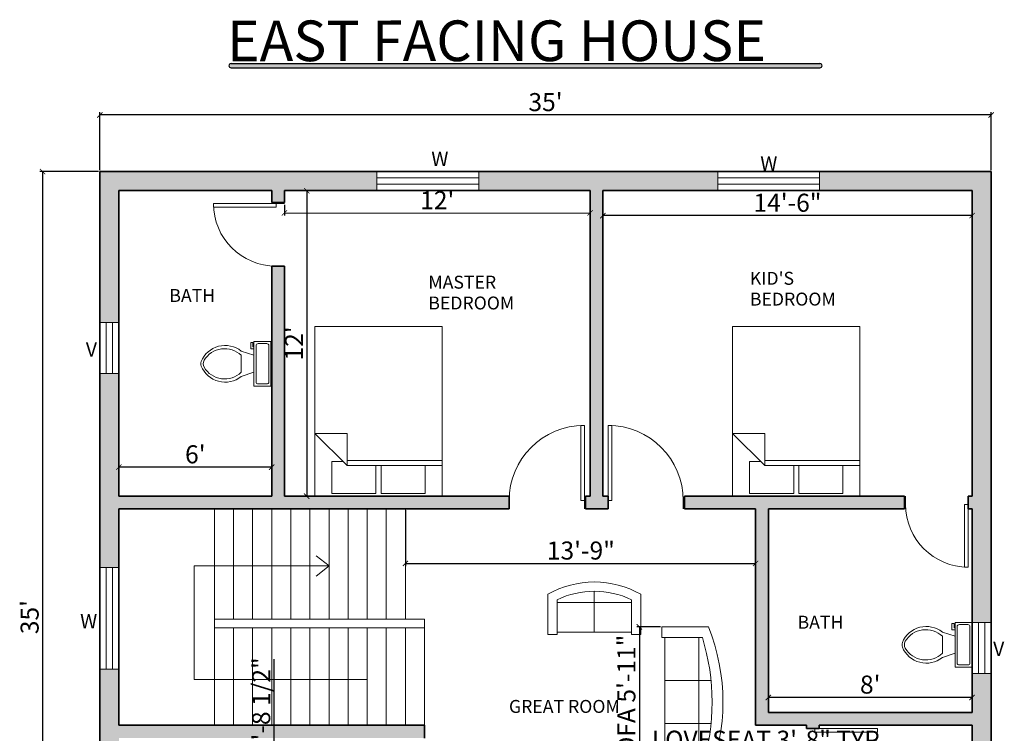
# Model space of a CAD drawing. Units: inches. Extents: x 3799 to 20199, y 1682 to 8087.
# Tile 5 of 30: x 8822 to 9286, y 2151 to 2487. Entities that reach past the tile are written whole.
import ezdxf

# ---------------------------------------------------------------- set-up
doc = ezdxf.new("R2010")
doc.units = ezdxf.units.IN
for name, color, linetype, lineweight in [('A-ANNO-DIMS', 2, 'Continuous', 18), ('A-ANNO-SYMB', 3, 'Continuous', 18), ('A-ANNO-TITL', 7, 'Continuous', 25), ('A-AREA-IDEN', 7, 'Continuous', 18), ('A-DOOR', 3, 'Continuous', 18), ('A-FLOR-FIXT', 9, 'Continuous', 18), ('A-FLOR-STRS', 41, 'Continuous', 18), ('A-FURN', 8, 'Continuous', 18), ('A-GLAZ', 152, 'Continuous', 18), ('A-WALL', 7, 'Continuous', 35), ('A-WALL-PATT', 252, 'Continuous', 13)]:
    doc.layers.add(name, color=color, linetype=linetype, lineweight=lineweight)
doc.styles.get("Standard").update_dxf_attribs({"font": 'arial.ttf'})
doc.dimstyles.new('ISO-25', dxfattribs={"dimtxt": 8.5, "dimasz": 2.5, "dimexe": 1.25, "dimexo": 0.625, "dimtad": 1, "dimdec": 0, "dimlunit": 3, "dimtxsty": 'Standard', "dimblk": 'ARCHTICK', "dimcen": 2.5, "dimadec": 0, "dimazin": 0, "dimtfac": 1, "dimtdec": 0, "dimtmove": 0, "dimatfit": 3, "dimfxl": 1, "dimarcsym": 0})

# ---------------------------------------------------------------- blocks, each defined once
blk = doc.blocks.new('*U16')
for p, q in [((0, 0), (0, -100)), ((900, 0), (900, -100))]:
    blk.add_line(p, q)
blk.add_lwpolyline([(0, 0), (0, 900), (43.75, 900), (43.75, 0)], close=True)
blk.add_arc((0, 0), 900, 0, 90)
blk = doc.blocks.new('*U21')
for p, q in [((9.5, -6), (9.5, -2)), ((-10, -8.5), (-8, -8.5)), ((-10, -9.5), (-10, -8.5)), ((-8, -8.5), (-8, -8)), ((-7, -8), (-7, -9.5)), ((-4, -8), (-6, -14)), ((4, -8), (6, -14)), ((-7, -9.5), (-10, -9.5)), ((4, -14), (-4, -14))]:
    blk.add_line(p, q)
blk.add_lwpolyline([(10.5, -8), (10.5, 0), (-10.5, 0), (-10.5, -8)], close=True)
for points in [[(-9.5, -2), (-9.5, -6)], [(8.5, -1), (-8.5, -1)], [(-8.5, -7), (8.5, -7)]]:
    blk.add_lwpolyline(points)
for centre, radius, start, end in [((-8.62, -1.88), 0.884, 81.8699, 188.1301), ((8.62, -1.88), 0.884, 351.8699, 98.1301), ((-8.62, -6.12), 0.884, 171.8699, 278.1301), ((8.62, -6.12), 0.884, 261.8699, 8.1301), ((3.52, -21.58), 12.17, 141.4691, 247.9714), ((4.2, -21.82), 11.33, 136.3677, 238.9468), ((-3.52, -21.58), 12.17, 292.0284, 38.5307), ((-4.2, -21.82), 11.33, 301.053, 43.6321), ((0, -27.88), 4, 245.7318, 294.2682), ((0, -29), 4, 254.8605, 285.1395)]:
    blk.add_arc(centre, radius, start, end)
blk = doc.blocks.new('*U22')
for p, q in [((0, 0), (0, -100)), ((-900, 0), (-900, -100))]:
    blk.add_line(p, q)
blk.add_lwpolyline([(0, 0), (0, 900), (-43.75, 900), (-43.75, 0)], close=True)
blk.add_arc((0, 0), 900, 90, 180)
blk = doc.blocks.new('*U17')
for p, q in [((-750, 0), (-750, -100)), ((0, 0), (0, -100))]:
    blk.add_line(p, q)
blk.add_lwpolyline([(0, 0), (0, 750), (-43.75, 750), (-43.75, 0)], close=True)
blk.add_arc((0, 0), 750, 90, 180)
blk = doc.blocks.new('*U7')
for p, q in [((0, 0), (0, -100)), ((750, 0), (750, -100))]:
    blk.add_line(p, q)
blk.add_lwpolyline([(0, 0), (0, 750), (43.75, 750), (43.75, 0)], close=True)
blk.add_arc((0, 0), 750, 0, 90)
blk = doc.blocks.new('*U24')
for p, q in [((-750, 0), (-750, 100)), ((0, 0), (0, 100))]:
    blk.add_line(p, q)
blk.add_lwpolyline([(0, 0), (0, -750), (-43.75, -750), (-43.75, 0)], close=True)
blk.add_arc((0, 0), 750, 180, 270)
blk = doc.blocks.new('Bed - Queen')
for p, q in [((0, -80.00003), (0, 0)), ((0, 0), (59.99999, 0)), ((59.99999, 0), (59.99999, -80.00003)), ((7.99999, -1.2), (28.79998, -1.2)), ((7.99999, -14.4), (7.99999, -1.2)), ((28.79998, -1.2), (28.79998, -14.4)), ((31.19999, -1.2), (51.99999, -1.2)), ((31.19999, -14.4), (31.19999, -1.2)), ((51.99999, -1.2), (51.99999, -16.4)), ((0, -14.4), (44.8, -14.4)), ((44.8, -16.8), (0, -16.8)), ((59.99999, -29.6), (44.8, -14.4)), ((44.8, -14.4), (44.8, -29.6)), ((51.99999, -16.4), (46.79936, -16.4)), ((44.8, -29.6), (59.99999, -29.6)), ((59.99999, -80.00003), (0, -80.00003))]:
    blk.add_line(p, q)
blk = doc.blocks.new('Sofa - Roundback 7 ft.')
for p, q in [((-12.00002, -32.4421), (-12.00003, -6.5971)), ((11.99997, -32.4421), (11.99998, -6.5971)), ((-36.000027, -34), (-36.000027, -11.4696)), ((-35.999844, -13.3819), (35.9998, -13.3819)), ((35.99998, -34), (35.99998, -11.4696)), ((-36.000027, -32.4421), (35.99998, -32.4421))]:
    blk.add_line(p, q)
for points in [[(-36.000027, -34), (-42.000027, -34), (-42.000027, -8)], [(41.99998, -8), (41.99998, -34), (35.99998, -34)]]:
    blk.add_lwpolyline(points)
for centre, radius, start, end in [((0, -114.25), 114.25, 68.43141, 111.5686), ((-0.00001, -127.1968), 121.1968, 72.72033, 107.2797)]:
    blk.add_arc(centre, radius, start, end)
blk = doc.blocks.new('Sofa - Roundback Loveseat 5 ft.')
for p, q in [((0, -32.44198), (0, -5.99998)), ((-24, -33.99998), (-24, -11.46958)), ((24.00004, -33.99998), (24.00004, -11.46958)), ((-23.9998, -13.38178), (23.99986, -13.38178)), ((-24, -32.44198), (24.00004, -32.44198))]:
    blk.add_line(p, q)
for points in [[(-24, -33.99998), (-30, -33.99998), (-30, -7.99998)], [(30.00004, -7.99998), (30.00004, -33.99998), (24.00004, -33.99998)]]:
    blk.add_lwpolyline(points)
for centre, radius, start, end in [((0, -60.24998), 60.24998, 60.13715, 119.8628), ((0, -61.38438), 55.38444, 64.32083, 115.6792)]:
    blk.add_arc(centre, radius, start, end)
blk = doc.blocks.new('_ArchTick')
at = {"color": 0, "linetype": 'ByBlock', "const_width": 0.15}
blk.add_lwpolyline([(-0.5, -0.5), (0.5, 0.5)], dxfattribs=at)
blk = doc.blocks.new('*D31')
at = {"layer": 'A-ANNO-DIMS', "color": 0, "lineweight": -2, "transparency": 16777216}
for p, q in [((8860.21, 2416.04), (8860.21, 2443.34)), ((9280.21, 2442.09), (8860.21, 2442.09)), ((9280.21, 2416.04), (9280.21, 2443.34))]:
    blk.add_line(p, q, dxfattribs=at)
at = {"layer": 'Defpoints', "color": 0, "transparency": 16777216}
for p in [(8860.21, 2442.09), (8860.21, 2415.42), (9280.21, 2415.42)]:
    blk.add_point(p, dxfattribs=at)
at = {"layer": 'A-ANNO-DIMS', "color": 0, "lineweight": -2, "transparency": 16777216, "xscale": 2.5, "yscale": 2.5, "zscale": 2.5, "rotation": 180}
blk.add_blockref('_ArchTick', (8860.21, 2442.09), dxfattribs=at)
at = {"layer": 'A-ANNO-DIMS', "color": 0, "lineweight": -2, "transparency": 16777216, "xscale": 2.5, "yscale": 2.5, "zscale": 2.5}
blk.add_blockref('_ArchTick', (9280.21, 2442.09), dxfattribs=at)
at = {"layer": 'A-ANNO-DIMS', "color": 0, "transparency": 16777216, "insert": (9070.21, 2447.06), "char_height": 8.5, "attachment_point": 5}
blk.add_mtext("35'", dxfattribs=at)
blk = doc.blocks.new('*D32')
at = {"layer": 'A-ANNO-DIMS', "color": 0, "lineweight": -2, "transparency": 16777216}
for p, q in [((8859.58, 2415.42), (8831.97, 2415.42)), ((8833.22, 2415.42), (8833.22, 1995.42)), ((8859.58, 1995.42), (8831.97, 1995.42))]:
    blk.add_line(p, q, dxfattribs=at)
at = {"layer": 'Defpoints', "color": 0, "transparency": 16777216}
for p in [(8860.21, 2415.42), (8833.22, 1995.42), (8860.21, 1995.42)]:
    blk.add_point(p, dxfattribs=at)
at = {"layer": 'A-ANNO-DIMS', "color": 0, "lineweight": -2, "transparency": 16777216, "xscale": 2.5, "yscale": 2.5, "zscale": 2.5}
for p, rotation in [((8833.22, 2415.42), 90), ((8833.22, 1995.42), 270)]:
    blk.add_blockref('_ArchTick', p, dxfattribs=dict(at, rotation=rotation))
at = {"layer": 'A-ANNO-DIMS', "color": 0, "transparency": 16777216, "insert": (8828.25, 2205.42), "char_height": 8.5, "attachment_point": 5, "rotation": 90}
blk.add_mtext("35'", dxfattribs=at)
blk = doc.blocks.new('*D33')
at = {"layer": 'A-ANNO-DIMS', "color": 0, "lineweight": -2, "transparency": 16777216}
for p, q in [((8869.21, 2263.04), (8869.21, 2277.34)), ((8941.21, 2276.09), (8869.21, 2276.09)), ((8941.21, 2263.04), (8941.21, 2277.34))]:
    blk.add_line(p, q, dxfattribs=at)
at = {"layer": 'Defpoints', "color": 0, "transparency": 16777216}
for p in [(8869.21, 2276.09), (8869.21, 2262.42), (8941.21, 2262.42)]:
    blk.add_point(p, dxfattribs=at)
at = {"layer": 'A-ANNO-DIMS', "color": 0, "lineweight": -2, "transparency": 16777216, "xscale": 2.5, "yscale": 2.5, "zscale": 2.5, "rotation": 180}
blk.add_blockref('_ArchTick', (8869.21, 2276.09), dxfattribs=at)
at = {"layer": 'A-ANNO-DIMS', "color": 0, "lineweight": -2, "transparency": 16777216, "xscale": 2.5, "yscale": 2.5, "zscale": 2.5}
blk.add_blockref('_ArchTick', (8941.21, 2276.09), dxfattribs=at)
at = {"layer": 'A-ANNO-DIMS', "color": 0, "transparency": 16777216, "insert": (8905.21, 2281.05), "char_height": 8.5, "attachment_point": 5}
blk.add_mtext("6'", dxfattribs=at)
blk = doc.blocks.new('*D34')
at = {"layer": 'A-ANNO-DIMS', "color": 0, "lineweight": -2, "transparency": 16777216}
for p, q in [((8947.83, 2406.42), (8958.95, 2406.42)), ((8957.7, 2406.42), (8957.7, 2262.42)), ((8947.83, 2262.42), (8958.95, 2262.42))]:
    blk.add_line(p, q, dxfattribs=at)
at = {"layer": 'Defpoints', "color": 0, "transparency": 16777216}
for p in [(8947.21, 2406.42), (8947.21, 2262.42), (8957.7, 2262.42)]:
    blk.add_point(p, dxfattribs=at)
at = {"layer": 'A-ANNO-DIMS', "color": 0, "lineweight": -2, "transparency": 16777216, "xscale": 2.5, "yscale": 2.5, "zscale": 2.5}
for p, rotation in [((8957.7, 2406.42), 90), ((8957.7, 2262.42), 270)]:
    blk.add_blockref('_ArchTick', p, dxfattribs=dict(at, rotation=rotation))
at = {"layer": 'A-ANNO-DIMS', "color": 0, "transparency": 16777216, "insert": (8952.81, 2334.42), "char_height": 8.5, "attachment_point": 5, "rotation": 90}
blk.add_mtext("12'", dxfattribs=at)
blk = doc.blocks.new('*D35')
at = {"layer": 'A-ANNO-DIMS', "color": 0, "lineweight": -2, "transparency": 16777216}
for p, q in [((8947.21, 2399.71), (8947.21, 2394.69)), ((9091.21, 2399.65), (9091.21, 2394.63)), ((8947.21, 2395.94), (9091.21, 2395.88))]:
    blk.add_line(p, q, dxfattribs=at)
at = {"layer": 'Defpoints', "color": 0, "transparency": 16777216}
for p in [(8947.21, 2400.33), (9091.21, 2400.28), (9091.21, 2395.88)]:
    blk.add_point(p, dxfattribs=at)
at = {"layer": 'A-ANNO-DIMS', "color": 0, "lineweight": -2, "transparency": 16777216, "xscale": 2.5, "yscale": 2.5, "zscale": 2.5}
for p, rotation in [((8947.21, 2395.94), 179.9775700857239), ((9091.21, 2395.88), 359.9775700857239)]:
    blk.add_blockref('_ArchTick', p, dxfattribs=dict(at, rotation=rotation))
at = {"layer": 'A-ANNO-DIMS', "color": 0, "transparency": 16777216, "insert": (9019.21, 2400.8), "char_height": 8.5, "attachment_point": 5, "rotation": 359.9776}
blk.add_mtext("12'", dxfattribs=at)
blk = doc.blocks.new('*D36')
at = {"layer": 'A-ANNO-DIMS', "color": 0, "lineweight": -2, "transparency": 16777216}
for p, q in [((9097.21, 2405.79), (9097.21, 2393.39)), ((9271.21, 2405.79), (9271.21, 2393.39)), ((9271.21, 2394.64), (9097.21, 2394.64))]:
    blk.add_line(p, q, dxfattribs=at)
at = {"layer": 'Defpoints', "color": 0, "transparency": 16777216}
for p in [(9097.21, 2406.42), (9271.21, 2406.42), (9097.21, 2394.64)]:
    blk.add_point(p, dxfattribs=at)
at = {"layer": 'A-ANNO-DIMS', "color": 0, "lineweight": -2, "transparency": 16777216, "xscale": 2.5, "yscale": 2.5, "zscale": 2.5, "rotation": 180}
blk.add_blockref('_ArchTick', (9097.21, 2394.64), dxfattribs=at)
at = {"layer": 'A-ANNO-DIMS', "color": 0, "lineweight": -2, "transparency": 16777216, "xscale": 2.5, "yscale": 2.5, "zscale": 2.5}
blk.add_blockref('_ArchTick', (9271.21, 2394.64), dxfattribs=at)
at = {"layer": 'A-ANNO-DIMS', "color": 0, "transparency": 16777216, "insert": (9184.21, 2399.61), "char_height": 8.5, "attachment_point": 5}
blk.add_mtext('14\'-6"', dxfattribs=at)
blk = doc.blocks.new('*D37')
at = {"layer": 'A-ANNO-DIMS', "color": 0, "lineweight": -2, "transparency": 16777216}
for p, q in [((9175.21, 2161.04), (9175.21, 2168.8)), ((9271.21, 2167.55), (9175.21, 2167.55)), ((9271.21, 2161.04), (9271.21, 2168.8))]:
    blk.add_line(p, q, dxfattribs=at)
at = {"layer": 'Defpoints', "color": 0, "transparency": 16777216}
for p in [(9175.21, 2167.55), (9175.21, 2160.42), (9271.21, 2160.42)]:
    blk.add_point(p, dxfattribs=at)
at = {"layer": 'A-ANNO-DIMS', "color": 0, "lineweight": -2, "transparency": 16777216, "xscale": 2.5, "yscale": 2.5, "zscale": 2.5, "rotation": 180}
blk.add_blockref('_ArchTick', (9175.21, 2167.55), dxfattribs=at)
at = {"layer": 'A-ANNO-DIMS', "color": 0, "lineweight": -2, "transparency": 16777216, "xscale": 2.5, "yscale": 2.5, "zscale": 2.5}
blk.add_blockref('_ArchTick', (9271.21, 2167.55), dxfattribs=at)
at = {"layer": 'A-ANNO-DIMS', "color": 0, "transparency": 16777216, "insert": (9223.21, 2172.52), "char_height": 8.5, "attachment_point": 5}
blk.add_mtext("8'", dxfattribs=at)
blk = doc.blocks.new('*D46')
at = {"layer": 'A-ANNO-DIMS', "color": 0, "lineweight": -2, "transparency": 16777216}
for p, q in [((9004.21, 2255.79), (9004.21, 2229.48)), ((9169.21, 2255.79), (9169.21, 2229.48)), ((9004.21, 2230.73), (9169.21, 2230.73))]:
    blk.add_line(p, q, dxfattribs=at)
at = {"layer": 'Defpoints', "color": 0, "transparency": 16777216}
for p in [(9004.21, 2256.42), (9169.21, 2256.42), (9169.21, 2230.73)]:
    blk.add_point(p, dxfattribs=at)
at = {"layer": 'A-ANNO-DIMS', "color": 0, "lineweight": -2, "transparency": 16777216, "xscale": 2.5, "yscale": 2.5, "zscale": 2.5, "rotation": 180}
blk.add_blockref('_ArchTick', (9004.21, 2230.73), dxfattribs=at)
at = {"layer": 'A-ANNO-DIMS', "color": 0, "lineweight": -2, "transparency": 16777216, "xscale": 2.5, "yscale": 2.5, "zscale": 2.5}
blk.add_blockref('_ArchTick', (9169.21, 2230.73), dxfattribs=at)
at = {"layer": 'A-ANNO-DIMS', "color": 0, "transparency": 16777216, "insert": (9086.87, 2235.7), "char_height": 8.5, "attachment_point": 5}
blk.add_mtext('13\'-9"', dxfattribs=at)
blk = doc.blocks.new('WIN-24IN-9IN-FRAME')
for p, q in [((0, 24), (9, 24)), ((3, 0), (3, 24)), ((6, 0), (6, 24)), ((0, 0), (9, 0))]:
    blk.add_line(p, q)
blk = doc.blocks.new('WIN-48IN-9IN-FRAME')
for p, q in [((0, 0), (0, 9)), ((48, 6), (0, 6)), ((48, 0), (48, 9)), ((48, 3), (0, 3))]:
    blk.add_line(p, q)
blk = doc.blocks.new('*D256')
at = {"layer": 'A-ANNO-DIMS', "color": 0, "lineweight": -2, "transparency": 16777216}
for p, q in [((9124.45, 2200.84), (9113.18, 2200.84)), ((9114.43, 2200.84), (9114.43, 2129.88)), ((9124.45, 2129.88), (9113.18, 2129.88))]:
    blk.add_line(p, q, dxfattribs=at)
at = {"layer": 'Defpoints', "color": 0, "transparency": 16777216}
for p in [(9125.08, 2200.84), (9114.43, 2129.88), (9125.08, 2129.88)]:
    blk.add_point(p, dxfattribs=at)
at = {"layer": 'A-ANNO-DIMS', "color": 0, "lineweight": -2, "transparency": 16777216, "xscale": 2.5, "yscale": 2.5, "zscale": 2.5}
for p, rotation in [((9114.43, 2200.84), 90), ((9114.43, 2129.88), 270)]:
    blk.add_blockref('_ArchTick', p, dxfattribs=dict(at, rotation=rotation))
at = {"layer": 'A-ANNO-DIMS', "color": 0, "transparency": 16777216, "insert": (9109.41, 2165.36), "char_height": 8.5, "attachment_point": 5, "rotation": 90}
blk.add_mtext('SOFA 5\'-11"', dxfattribs=at)
blk = doc.blocks.new('*D274')
at = {"layer": 'A-ANNO-DIMS', "color": 0, "lineweight": -2, "transparency": 16777216}
for p, q in [((9070, 2135.57), (9070, 2142.76)), ((9070, 2141.51), (9113.8, 2141.51)), ((9113.8, 2135.57), (9113.8, 2142.76)), ((9113.8, 2141.51), (9234.98, 2141.51))]:
    blk.add_line(p, q, dxfattribs=at)
at = {"layer": 'Defpoints', "color": 0, "transparency": 16777216}
for p in [(9113.8, 2141.51), (9070, 2134.94), (9113.8, 2134.94)]:
    blk.add_point(p, dxfattribs=at)
at = {"layer": 'A-ANNO-DIMS', "color": 0, "lineweight": -2, "transparency": 16777216, "xscale": 2.5, "yscale": 2.5, "zscale": 2.5, "rotation": 180}
blk.add_blockref('_ArchTick', (9070, 2141.51), dxfattribs=at)
at = {"layer": 'A-ANNO-DIMS', "color": 0, "lineweight": -2, "transparency": 16777216, "xscale": 2.5, "yscale": 2.5, "zscale": 2.5}
blk.add_blockref('_ArchTick', (9113.8, 2141.51), dxfattribs=at)
at = {"layer": 'A-ANNO-DIMS', "color": 0, "transparency": 16777216, "insert": (9175.64, 2146.54), "char_height": 8.5, "attachment_point": 5}
blk.add_mtext('LOVESEAT 3\'-8" TYP.', dxfattribs=at)
blk = doc.blocks.new('*D289')
at = {"layer": 'A-ANNO-DIMS', "color": 0, "lineweight": -2, "transparency": 16777216}
for p, q in [((8942.35, 2139.27), (8942.35, 2185.57)), ((8934.89, 2139.27), (8943.6, 2139.27)), ((8942.35, 2106.67), (8942.35, 2139.27)), ((8934.89, 2106.67), (8943.6, 2106.67))]:
    blk.add_line(p, q, dxfattribs=at)
at = {"layer": 'Defpoints', "color": 0, "transparency": 16777216}
for p in [(8934.26, 2139.27), (8942.35, 2139.27), (8934.26, 2106.67)]:
    blk.add_point(p, dxfattribs=at)
at = {"layer": 'A-ANNO-DIMS', "color": 0, "lineweight": -2, "transparency": 16777216, "xscale": 2.5, "yscale": 2.5, "zscale": 2.5}
for p, rotation in [((8942.35, 2139.27), 90), ((8942.35, 2106.67), 270)]:
    blk.add_blockref('_ArchTick', p, dxfattribs=dict(at, rotation=rotation))
at = {"layer": 'A-ANNO-DIMS', "color": 0, "transparency": 16777216, "insert": (8937.34, 2163.67), "char_height": 8.5, "attachment_point": 5, "rotation": 90}
blk.add_mtext('2\'-8 1/2"', dxfattribs=at)

msp = doc.modelspace()

# ---------------------------------------------------------------- hatches: boundary and pattern name
at = {"layer": 'A-ANNO-TITL'}
h = msp.add_hatch(color=256, dxfattribs=at)
h.dxf.hatch_style = 1
h.paths.add_polyline_path([(9199.52, 2466.32), (8922.06, 2466.32, 1), (8922.06, 2464.32), (9199.52, 2464.32, 1)])
at = {"layer": 'A-WALL-PATT'}
h = msp.add_hatch(color=256, dxfattribs=at)
h.dxf.hatch_style = 1
h.paths.add_polyline_path([(8869.21, 2406.42), (8941.21, 2406.42), (8941.21, 2400.8), (8947.21, 2400.8), (8947.21, 2406.42), (8990.79, 2406.42), (8990.79, 2415.42), (8860.21, 2415.42), (8860.21, 2344.29), (8869.21, 2344.29)])
h.paths.add_polyline_path([(8869.21, 2320.29), (8860.21, 2320.29), (8860.21, 2228.85), (8869.21, 2228.85), (8869.21, 2256.42), (9053.08, 2256.42), (9053.08, 2262.42), (8947.21, 2262.42), (8947.21, 2370.8), (8941.21, 2370.8), (8941.21, 2262.42), (8869.21, 2262.42)])
h.paths.add_polyline_path([(9151.38, 2415.42), (9038.79, 2415.42), (9038.79, 2406.42), (9091.21, 2406.42), (9091.21, 2262.42), (9089.08, 2262.42), (9089.08, 2256.42), (9097.21, 2256.42), (9099.67, 2256.42), (9099.67, 2262.42), (9097.21, 2262.42), (9097.21, 2406.42), (9151.38, 2406.42)])
h.paths.add_polyline_path([(9280.21, 2415.42), (9199.38, 2415.42), (9199.38, 2406.42), (9271.21, 2406.42), (9271.21, 2262.42), (9269.42, 2262.42), (9269.42, 2256.42), (9271.21, 2256.42), (9271.21, 2202.87), (9280.21, 2202.87)])
h.paths.add_polyline_path([(9280.21, 2178.87), (9271.21, 2178.87), (9271.21, 2160.42), (9175.21, 2160.42), (9175.21, 2256.42), (9239.42, 2256.42), (9239.42, 2262.42), (9135.67, 2262.42), (9135.67, 2256.42), (9169.21, 2256.42), (9169.21, 2154.42), (9193.21, 2154.42), (9193.21, 2152.89), (9199.21, 2152.89), (9199.21, 2154.42), (9271.21, 2154.42), (9271.21, 2120.19), (9280.21, 2120.19)])
h.paths.add_polyline_path([(9199.21, 2122.89), (9193.21, 2122.89), (9193.21, 2082.42), (9199.21, 2082.42)])
h.paths.add_polyline_path([(9146.43, 2004.42), (9127.21, 2004.42), (9127.21, 2076.42), (9121.21, 2076.42), (9121.21, 2004.42), (9106.79, 2004.42), (9106.79, 1995.42), (9146.43, 1995.42)])
h.paths.add_polyline_path([(9058.79, 2004.42), (9049.21, 2004.42), (9049.21, 2082.42), (9041.72, 2082.42), (9041.72, 2076.42), (9043.21, 2076.42), (9043.21, 2004.42), (9032.46, 2004.42), (9032.46, 1995.42), (9058.79, 1995.42)])
h.paths.add_polyline_path([(8984.46, 2004.42), (8971.21, 2004.42), (8971.21, 2076.42), (9011.72, 2076.42), (9011.72, 2082.42), (8965.21, 2082.42), (8965.21, 2004.42), (8931.73, 2004.42), (8931.73, 1995.42), (8984.46, 1995.42)])
h.paths.add_polyline_path([(8883.73, 2004.42), (8869.21, 2004.42), (8869.21, 2064.88), (8860.21, 2064.88), (8860.21, 1995.42), (8883.73, 1995.42)])
h.paths.add_polyline_path([(8869.21, 2148.42), (9013.21, 2148.42), (9013.21, 2154.42), (8869.21, 2154.42), (8869.21, 2180.85), (8860.21, 2180.85), (8860.21, 2112.88), (8869.21, 2112.88)])

# ---------------------------------------------------------------- linework, layer by layer
at = {"layer": 'A-ANNO-TITL'}
for p, q in [((8922.06, 2466.32), (9199.52, 2466.32)), ((8922.06, 2464.32), (9199.52, 2464.32))]:
    msp.add_line(p, q, dxfattribs=at)
for centre, start, end in [((8922.06, 2465.32), 90, 270), ((9199.52, 2465.32), 270, 90)]:
    msp.add_arc(centre, 1, start, end, dxfattribs=at)
at = {"layer": 'A-FLOR-STRS'}
for p, q in [((8914.21, 2154.42), (8914.21, 2256.42)), ((8923.21, 2204.42), (8923.21, 2256.42)), ((8932.21, 2204.42), (8932.21, 2256.42)), ((8941.21, 2204.42), (8941.21, 2256.42)), ((8950.21, 2204.42), (8950.21, 2256.42)), ((8959.21, 2204.42), (8959.21, 2256.42)), ((8968.21, 2204.42), (8968.21, 2256.42)), ((8977.21, 2204.42), (8977.21, 2256.42)), ((8986.21, 2204.42), (8986.21, 2256.42)), ((8995.21, 2204.42), (8995.21, 2256.42)), ((9004.21, 2204.42), (9004.21, 2256.42)), ((8968.21, 2229.52), (8962.15, 2234.32)), ((8904.62, 2176.03), (8904.62, 2229.52)), ((8904.62, 2229.52), (8968.21, 2229.52)), ((8968.21, 2229.52), (8962.15, 2224.72)), ((9013.21, 2204.42), (8914.21, 2204.42)), ((9013.21, 2154.42), (9013.21, 2204.42)), ((9013.21, 2200.42), (8914.21, 2200.42)), ((8923.21, 2154.42), (8923.21, 2200.42)), ((8932.21, 2154.42), (8932.21, 2200.42)), ((8941.21, 2154.42), (8941.21, 2200.42)), ((8950.21, 2154.42), (8950.21, 2200.42)), ((8959.21, 2154.42), (8959.21, 2200.42)), ((8968.21, 2154.42), (8968.21, 2200.42)), ((8977.21, 2154.42), (8977.21, 2200.42)), ((8986.21, 2154.42), (8986.21, 2200.42)), ((8995.21, 2154.42), (8995.21, 2200.42)), ((9004.21, 2154.42), (9004.21, 2200.42)), ((8986.21, 2176.03), (8904.62, 2176.03))]:
    msp.add_line(p, q, dxfattribs=at)
at = {"layer": 'A-WALL'}
for p, q in [((9280.21, 2415.42), (8860.21, 2415.42)), ((8860.21, 2415.42), (8860.21, 1995.42)), ((9280.21, 1995.42), (9280.21, 2415.42)), ((8869.21, 2406.42), (8869.21, 2262.42)), ((8941.21, 2406.42), (8869.21, 2406.42)), ((8941.21, 2406.42), (8941.21, 2400.8)), ((8947.21, 2406.42), (8947.21, 2400.8)), ((9091.21, 2406.42), (8947.21, 2406.42)), ((9091.21, 2406.42), (9091.21, 2262.42)), ((9271.21, 2406.42), (9097.21, 2406.42)), ((9097.21, 2406.42), (9097.21, 2262.42)), ((9271.21, 2262.42), (9271.21, 2406.42)), ((8941.21, 2400.8), (8947.21, 2400.8)), ((8941.21, 2370.8), (8947.21, 2370.8)), ((8941.21, 2370.8), (8941.21, 2262.42)), ((8947.21, 2370.8), (8947.21, 2262.42)), ((8941.21, 2262.42), (8869.21, 2262.42)), ((9053.08, 2262.42), (8947.21, 2262.42)), ((9053.08, 2262.42), (9053.08, 2256.42)), ((9091.21, 2262.42), (9089.08, 2262.42)), ((9089.08, 2262.42), (9089.08, 2256.42)), ((9099.67, 2262.42), (9097.21, 2262.42)), ((9099.67, 2262.42), (9099.67, 2256.42)), ((9135.67, 2262.42), (9135.67, 2256.42)), ((9239.42, 2262.42), (9135.67, 2262.42)), ((9239.42, 2256.42), (9239.42, 2262.42)), ((9271.21, 2262.42), (9269.42, 2262.42)), ((9269.42, 2256.42), (9269.42, 2262.42)), ((8869.21, 2256.42), (8869.21, 2154.42)), ((9053.08, 2256.42), (8869.21, 2256.42)), ((9097.21, 2256.42), (9089.08, 2256.42)), ((9099.67, 2256.42), (9097.21, 2256.42)), ((9169.21, 2256.42), (9135.67, 2256.42)), ((9169.21, 2154.42), (9169.21, 2256.42)), ((9175.21, 2160.42), (9175.21, 2256.42)), ((9239.42, 2256.42), (9175.21, 2256.42)), ((9271.21, 2256.42), (9269.42, 2256.42)), ((9271.21, 2160.42), (9271.21, 2256.42)), ((9271.21, 2160.42), (9175.21, 2160.42)), ((9013.21, 2154.42), (8869.21, 2154.42)), ((9013.21, 2148.42), (9013.21, 2154.42)), ((9193.21, 2154.42), (9169.21, 2154.42)), ((9193.21, 2152.89), (9193.21, 2154.42)), ((9193.21, 2152.89), (9199.21, 2152.89)), ((9271.21, 2154.42), (9199.21, 2154.42)), ((9199.21, 2152.89), (9199.21, 2154.42)), ((9271.21, 2082.42), (9271.21, 2154.42))]:
    msp.add_line(p, q, dxfattribs=at)

# ---------------------------------------------------------------- block references
at = {"layer": 'A-DOOR', "xscale": 0.0393700787401575, "yscale": 0.0393700787401575, "zscale": 0.0393700787401575}
for name, p, rotation in [('*U17', (8943.27, 2400.33), 90), ('*U7', (9197.15, 2152.89), 270)]:
    msp.add_blockref(name, p, dxfattribs=dict(at, rotation=rotation))
for name, p in [('*U22', (9088.51, 2260.36)), ('*U16', (9099.67, 2260.36)), ('*U24', (9269.42, 2258.48))]:
    msp.add_blockref(name, p, dxfattribs=at)
at = {"layer": 'A-FLOR-FIXT', "rotation": 270}
for p in [(8940.85, 2324.81), (9271.21, 2192.37)]:
    msp.add_blockref('*U21', p, dxfattribs=at)
at = {"layer": 'A-FURN', "rotation": 180}
for p in [(9021.54, 2262.42), (9218.37, 2262.42)]:
    msp.add_blockref('Bed - Queen', p, dxfattribs=at)
at = {"layer": 'A-FURN', "xscale": 0.729884385846111, "yscale": 0.729884385846111, "zscale": 0.729884385846111}
msp.add_blockref('Sofa - Roundback Loveseat 5 ft.', (9093.22, 2222), dxfattribs=at)
at = {"layer": 'A-FURN', "xscale": 0.8447815510693718, "yscale": 0.8447815510693718, "zscale": 0.8447815510693718, "rotation": 270}
msp.add_blockref('Sofa - Roundback 7 ft.', (9153.8, 2165.36), dxfattribs=at)
at = {"layer": 'A-GLAZ'}
for name, p in [('WIN-48IN-9IN-FRAME', (8990.79, 2406.42)), ('WIN-48IN-9IN-FRAME', (9151.38, 2406.42)), ('WIN-24IN-9IN-FRAME', (8860.21, 2320.29)), ('WIN-24IN-9IN-FRAME', (9271.21, 2178.87))]:
    msp.add_blockref(name, p, dxfattribs=at)
at = {"layer": 'A-GLAZ', "rotation": 90}
msp.add_blockref('WIN-48IN-9IN-FRAME', (8869.21, 2180.85), dxfattribs=at)

# ---------------------------------------------------------------- texts
at = {"layer": 'A-ANNO-SYMB'}
for s, p in [('W', (9016.42, 2418.05)), ('W', (9171.42, 2415.88)), ('V', (8853.62, 2328.24)), ('W', (8850.95, 2200.16)), ('V', (9281.13, 2187.14))]:
    msp.add_text(s, height=6.71, rotation=0.0167, dxfattribs=at).set_placement(p)
at = {"layer": 'A-ANNO-TITL'}
msp.add_text('EAST FACING HOUSE', height=19.1524, rotation=0.0167, dxfattribs=at).set_placement((8920.12, 2467.44))
at = {"layer": 'A-AREA-IDEN'}
for s, p in [('MASTER', (9015.01, 2360.22)), ("KID'S", (9166.51, 2362.05)), ('BATH', (8892.99, 2353.95)), ('BEDROOM', (9166.51, 2352.25)), ('BEDROOM', (9015.01, 2350.42)), ('BATH', (9188.97, 2199.96)), ('GREAT ROOM', (9053, 2160.27))]:
    msp.add_text(s, height=6.1, rotation=0.0167, dxfattribs=at).set_placement(p)

# ---------------------------------------------------------------- dimensions: what is measured, and where the dimension line sits
at = {"layer": 'A-ANNO-DIMS'}
for base, p1, p2, picture, middle in [((8860.21, 2442.09), (9280.21, 2415.42), (8860.21, 2415.42), '*D31', (9070.21, 2447.06)), ((9097.21, 2394.64), (9271.21, 2406.42), (9097.21, 2406.42), '*D36', (9184.21, 2399.61)), ((8869.21, 2276.09), (8941.21, 2262.42), (8869.21, 2262.42), '*D33', (8905.21, 2281.05)), ((9175.21, 2167.55), (9271.21, 2160.42), (9175.21, 2160.42), '*D37', (9223.21, 2172.52))]:
    dim = msp.add_linear_dim(base=base, p1=p1, p2=p2, dimstyle='ISO-25', override={"dimclrd": 0, "dimclre": 0, "dimclrt": 0}, dxfattribs=at)
    dim.commit()
    dim.dimension.update_dxf_attribs({"geometry": picture, "text_midpoint": middle})
for base, p1, p2, override, picture, middle in [((8833.22, 1995.42), (8860.21, 2415.42), (8860.21, 1995.42), {"dimclrd": 0, "dimclre": 0, "dimclrt": 0}, '*D32', (8828.25, 2205.42)), ((8957.7, 2262.42), (8947.21, 2406.42), (8947.21, 2262.42), {"dimclrd": 0, "dimclre": 0, "dimclrt": 0}, '*D34', (8952.81, 2334.42)), ((8942.35, 2139.27), (8934.26, 2106.67), (8934.26, 2139.27), {"dimdec": 1, "dimlfac": 1, "dimrnd": 0, "dimzin": 1, "dimdsep": 46, "dimlunit": 4, "dimfrac": 2}, '*D289', (8937.34, 2163.67))]:
    dim = msp.add_linear_dim(base=base, p1=p1, p2=p2, angle=90, dimstyle='ISO-25', override=override, dxfattribs=at)
    dim.commit()
    dim.dimension.update_dxf_attribs({"geometry": picture, "text_midpoint": middle})
dim = msp.add_aligned_dim(p1=(8947.21, 2400.33), p2=(9091.21, 2400.28), distance=-4.39, dimstyle='ISO-25', override={"dimclrd": 0, "dimclre": 0, "dimclrt": 0}, dxfattribs=at)
dim.commit()
dim.dimension.update_dxf_attribs({"geometry": '*D35', "text_midpoint": (9019.21, 2400.8)})
dim = msp.add_linear_dim(base=(9169.21, 2230.73), p1=(9004.21, 2256.42), p2=(9169.21, 2256.42), dimstyle='ISO-25', override={"dimclrd": 0, "dimclre": 0, "dimclrt": 0}, dxfattribs=at)
dim.commit()
dim.dimension.update_dxf_attribs({"geometry": '*D46', "text_midpoint": (9086.87, 2230.73), "dimtype": 160})
dim = msp.add_linear_dim(base=(9114.43, 2129.88), p1=(9125.08, 2200.84), p2=(9125.08, 2129.88), angle=270, text='SOFA <>', dimstyle='ISO-25', override={"dimdec": 1, "dimlfac": 1, "dimrnd": 0, "dimzin": 1, "dimdsep": 46, "dimlunit": 4, "dimfrac": 2}, dxfattribs=at)
dim.commit()
dim.dimension.update_dxf_attribs({"geometry": '*D256', "text_midpoint": (9109.41, 2165.36)})
dim = msp.add_linear_dim(base=(9113.8, 2141.51), p1=(9070, 2134.94), p2=(9113.8, 2134.94), text='LOVESEAT <> TYP.', dimstyle='ISO-25', override={"dimdec": 1, "dimlfac": 1, "dimrnd": 0, "dimzin": 1, "dimdsep": 46, "dimlunit": 4, "dimfrac": 2}, dxfattribs=at)
dim.commit()
dim.dimension.update_dxf_attribs({"geometry": '*D274', "text_midpoint": (9175.64, 2146.54)})

doc.saveas('drawing.dxf')
